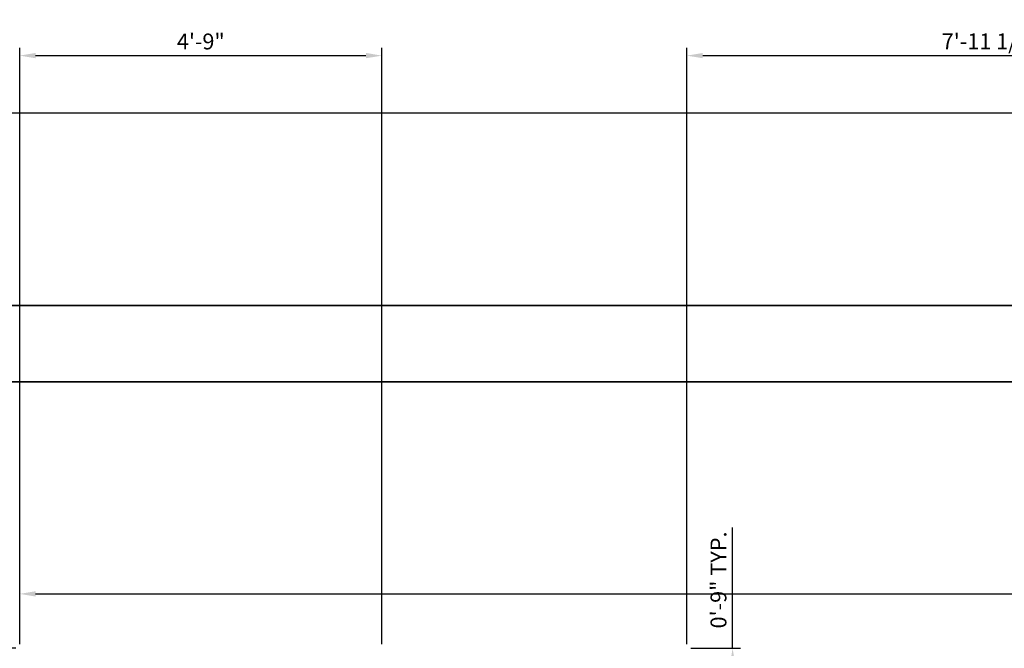
# Model space of a CAD drawing. Units: inches. Extents: x 2901 to 5923, y 918 to 2827.
# Tile 8 of 16: x 4430 to 4585, y 1630 to 1729. Entities that reach past the tile are written whole.
import ezdxf

# ---------------------------------------------------------------- set-up
doc = ezdxf.new("R2010")
doc.units = ezdxf.units.IN
doc.layers.add('A-ANNO-DIMS', color=2, linetype='Continuous', lineweight=18)
doc.layers.add('C-PROP', color=7, linetype='Continuous', lineweight=35)
doc.styles.get("Standard").update_dxf_attribs({"font": 'arial.ttf'})
doc.dimstyles.new('Copy of ISO-25', dxfattribs={"dimtxt": 2.5, "dimasz": 2.5, "dimexe": 1.25, "dimexo": 0.625, "dimtad": 1, "dimdec": 1, "dimlunit": 4, "dimtxsty": 'Standard', "dimcen": 2.5, "dimadec": 0, "dimazin": 0, "dimtfac": 1, "dimtdec": 1, "dimtmove": 0, "dimatfit": 3, "dimfxl": 1, "dimarcsym": 0})

# ---------------------------------------------------------------- blocks, each defined once
blk = doc.blocks.new('*D25')
at = {"layer": 'A-ANNO-DIMS', "color": 0, "lineweight": -2, "transparency": 16777216}
for p, q in [((4288.18, 1684.92), (4288.18, 1715.87)), ((5015.18, 1684.92), (5015.18, 1715.87)), ((4290.68, 1714.62), (5012.68, 1714.62))]:
    blk.add_line(p, q, dxfattribs=at)
at = {"layer": 'A-ANNO-DIMS', "color": 0, "transparency": 16777216}
for points in [[(4290.68, 1715.04), (4290.68, 1714.2), (4288.18, 1714.62)], [(5012.68, 1715.04), (5012.68, 1714.2), (5015.18, 1714.62)]]:
    blk.add_solid(points, dxfattribs=at)
at = {"layer": 'Defpoints', "color": 0, "transparency": 16777216}
for p in [(5015.18, 1714.62), (4288.18, 1684.29), (5015.18, 1684.29)]:
    blk.add_point(p, dxfattribs=at)
at = {"layer": 'A-ANNO-DIMS', "color": 0, "transparency": 16777216, "insert": (4651.68, 1716.52), "char_height": 2.5, "attachment_point": 5}
blk.add_mtext('60\'-7"', dxfattribs=at)
blk = doc.blocks.new('*D26')
at = {"layer": 'A-ANNO-DIMS', "color": 0, "lineweight": -2, "transparency": 16777216}
for p, q in [((4425.95, 1632.9), (4425.95, 1639.52)), ((4429.44, 1630.4), (4424.7, 1630.4)), ((4429.44, 1630.4), (4424.7, 1630.4)), ((4425.95, 1627.9), (4425.95, 1625.4))]:
    blk.add_line(p, q, dxfattribs=at)
at = {"layer": 'A-ANNO-DIMS', "color": 0, "transparency": 16777216}
for points in [[(4425.54, 1632.9), (4426.37, 1632.9), (4425.95, 1630.4)], [(4425.54, 1627.9), (4426.37, 1627.9), (4425.95, 1630.4)]]:
    blk.add_solid(points, dxfattribs=at)
at = {"layer": 'Defpoints', "color": 0, "transparency": 16777216}
for p in [(4425.95, 1630.4), (4430.07, 1630.4), (4430.07, 1630.4)]:
    blk.add_point(p, dxfattribs=at)
at = {"layer": 'A-ANNO-DIMS', "color": 0, "transparency": 16777216, "insert": (4424.05, 1637.46), "char_height": 2.5, "attachment_point": 5, "rotation": 90}
blk.add_mtext('0"', dxfattribs=at)
blk = doc.blocks.new('*D36')
at = {"layer": 'A-ANNO-DIMS', "color": 0, "lineweight": -2, "transparency": 16777216}
for p, q in [((4430.07, 1631.02), (4430.07, 1640.2)), ((4892.07, 1631.02), (4892.07, 1640.2)), ((4432.57, 1638.95), (4889.57, 1638.95))]:
    blk.add_line(p, q, dxfattribs=at)
at = {"layer": 'A-ANNO-DIMS', "color": 0, "transparency": 16777216}
for points in [[(4432.57, 1639.37), (4432.57, 1638.53), (4430.07, 1638.95)], [(4889.57, 1639.37), (4889.57, 1638.53), (4892.07, 1638.95)]]:
    blk.add_solid(points, dxfattribs=at)
at = {"layer": 'Defpoints', "color": 0, "transparency": 16777216}
for p in [(4892.07, 1638.95), (4430.07, 1630.4), (4892.07, 1630.4)]:
    blk.add_point(p, dxfattribs=at)
at = {"layer": 'A-ANNO-DIMS', "color": 0, "transparency": 16777216, "insert": (4661.07, 1640.85), "char_height": 2.5, "attachment_point": 5}
blk.add_mtext('38\'-6"', dxfattribs=at)
blk = doc.blocks.new('*D76')
at = {"layer": 'A-ANNO-DIMS', "color": 0, "lineweight": -2, "transparency": 16777216}
for p, q in [((4542.27, 1630.4), (4542.27, 1649.39)), ((4535.69, 1630.4), (4543.52, 1630.4)), ((4542.27, 1623.9), (4542.27, 1627.9)), ((4535.69, 1621.4), (4543.52, 1621.4))]:
    blk.add_line(p, q, dxfattribs=at)
at = {"layer": 'A-ANNO-DIMS', "color": 0, "transparency": 16777216}
for points in [[(4541.85, 1627.9), (4542.69, 1627.9), (4542.27, 1630.4)], [(4541.85, 1623.9), (4542.69, 1623.9), (4542.27, 1621.4)]]:
    blk.add_solid(points, dxfattribs=at)
at = {"layer": 'Defpoints', "color": 0, "transparency": 16777216}
for p in [(4535.07, 1630.4), (4542.27, 1630.4), (4535.07, 1621.4)]:
    blk.add_point(p, dxfattribs=at)
at = {"layer": 'A-ANNO-DIMS', "color": 0, "transparency": 16777216, "insert": (4540.37, 1641.14), "char_height": 2.5, "attachment_point": 5, "rotation": 90}
blk.add_mtext('0\'-9" TYP.', dxfattribs=at)
blk = doc.blocks.new('*D92')
at = {"layer": 'A-ANNO-DIMS', "color": 0, "lineweight": -2, "transparency": 16777216}
for p, q in [((4430.07, 1631.02), (4430.07, 1724.84)), ((4487.07, 1631.02), (4487.07, 1724.84)), ((4432.57, 1723.59), (4484.57, 1723.59))]:
    blk.add_line(p, q, dxfattribs=at)
at = {"layer": 'A-ANNO-DIMS', "color": 0, "transparency": 16777216}
for points in [[(4432.57, 1724.01), (4432.57, 1723.18), (4430.07, 1723.59)], [(4484.57, 1724.01), (4484.57, 1723.18), (4487.07, 1723.59)]]:
    blk.add_solid(points, dxfattribs=at)
at = {"layer": 'Defpoints', "color": 0, "transparency": 16777216}
for p in [(4487.07, 1723.59), (4430.07, 1630.4), (4487.07, 1630.4)]:
    blk.add_point(p, dxfattribs=at)
at = {"layer": 'A-ANNO-DIMS', "color": 0, "transparency": 16777216, "insert": (4458.57, 1725.49), "char_height": 2.5, "attachment_point": 5}
blk.add_mtext('4\'-9"', dxfattribs=at)
blk = doc.blocks.new('*D93')
at = {"layer": 'A-ANNO-DIMS', "color": 0, "lineweight": -2, "transparency": 16777216}
for p, q in [((4535.07, 1631.02), (4535.07, 1724.84)), ((4630.61, 1631.02), (4630.61, 1724.84)), ((4537.57, 1723.59), (4628.11, 1723.59))]:
    blk.add_line(p, q, dxfattribs=at)
at = {"layer": 'A-ANNO-DIMS', "color": 0, "transparency": 16777216}
for points in [[(4537.57, 1724.01), (4537.57, 1723.18), (4535.07, 1723.59)], [(4628.11, 1724.01), (4628.11, 1723.18), (4630.61, 1723.59)]]:
    blk.add_solid(points, dxfattribs=at)
at = {"layer": 'Defpoints', "color": 0, "transparency": 16777216}
for p in [(4630.61, 1723.59), (4535.07, 1630.4), (4630.61, 1630.4)]:
    blk.add_point(p, dxfattribs=at)
at = {"layer": 'A-ANNO-DIMS', "color": 0, "transparency": 16777216, "insert": (4582.84, 1725.51), "char_height": 2.5, "attachment_point": 5}
blk.add_mtext('7\'-11 1/2"', dxfattribs=at)

msp = doc.modelspace()

# ---------------------------------------------------------------- linework, layer by layer
at = {"layer": 'C-PROP'}
msp.add_lwpolyline([(4288.18, 1684.29), (5015.18, 1684.29), (5015.18, 958.29), (4288.18, 958.29)], close=True, dxfattribs=at)
msp.add_lwpolyline([(5003.18, 978.26), (5003.18, 970.29), (4300.18, 970.29), (4300.18, 1672.29), (5003.18, 1672.29), (5003.18, 1132.27)], dxfattribs=at)

# ---------------------------------------------------------------- dimensions: what is measured, and where the dimension line sits
at = {"layer": 'A-ANNO-DIMS'}
for base, p1, p2, override, picture, middle in [((4630.61, 1723.59), (4535.07, 1630.4), (4630.61, 1630.4), {"dimdec": 1, "dimlfac": 1, "dimrnd": 0, "dimzin": 1, "dimdsep": 46, "dimlunit": 4, "dimfrac": 2}, '*D93', (4582.84, 1725.51)), ((4487.07, 1723.59), (4430.07, 1630.4), (4487.07, 1630.4), {"dimdec": 1, "dimlfac": 1, "dimrnd": 0, "dimzin": 1, "dimdsep": 46, "dimlunit": 4, "dimfrac": 2}, '*D92', (4458.57, 1725.49)), ((5015.18, 1714.62), (4288.18, 1684.29), (5015.18, 1684.29), {"dimclrd": 0, "dimclre": 0, "dimclrt": 0}, '*D25', (4651.68, 1716.52)), ((4892.07, 1638.95), (4430.07, 1630.4), (4892.07, 1630.4), {"dimclrd": 0, "dimclre": 0, "dimclrt": 0}, '*D36', (4661.07, 1640.85))]:
    dim = msp.add_linear_dim(base=base, p1=p1, p2=p2, dimstyle='Copy of ISO-25', override=override, dxfattribs=at)
    dim.commit()
    dim.dimension.update_dxf_attribs({"geometry": picture, "text_midpoint": middle})
dim = msp.add_linear_dim(base=(4542.27, 1630.4), p1=(4535.07, 1621.4), p2=(4535.07, 1630.4), angle=90, text='<> TYP.', dimstyle='Copy of ISO-25', override={"dimdec": 1, "dimlfac": 1, "dimrnd": 0, "dimzin": 1, "dimdsep": 46, "dimlunit": 4, "dimfrac": 2}, dxfattribs=at)
dim.commit()
dim.dimension.update_dxf_attribs({"geometry": '*D76', "text_midpoint": (4540.37, 1641.14)})
dim = msp.add_linear_dim(base=(4425.95179115, 1630.39662355), p1=(4430.0684223, 1630.39662355), p2=(4430.0684223, 1630.39662355), angle=90, dimstyle='Copy of ISO-25', override={"dimclrd": 0, "dimclre": 0, "dimclrt": 0}, dxfattribs=at)
dim.commit()
dim.dimension.update_dxf_attribs({"geometry": '*D26', "text_midpoint": (4424.05035868, 1637.45835615)})

doc.saveas('drawing.dxf')
